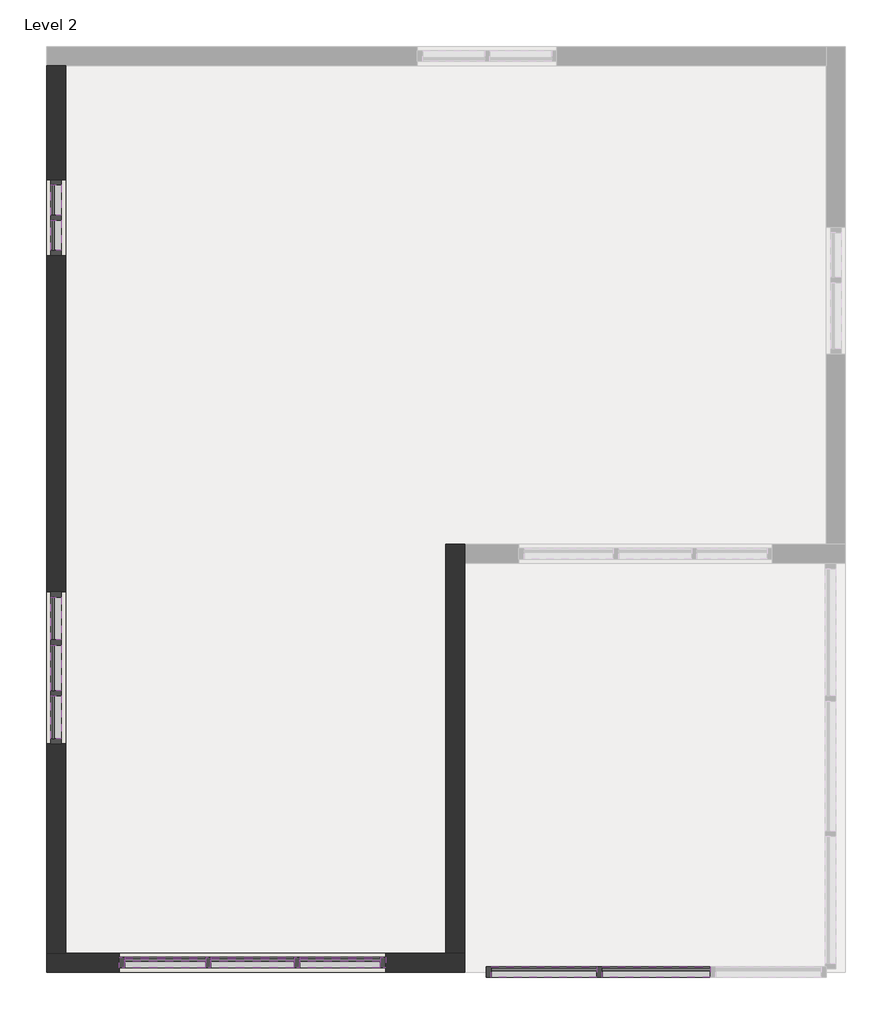
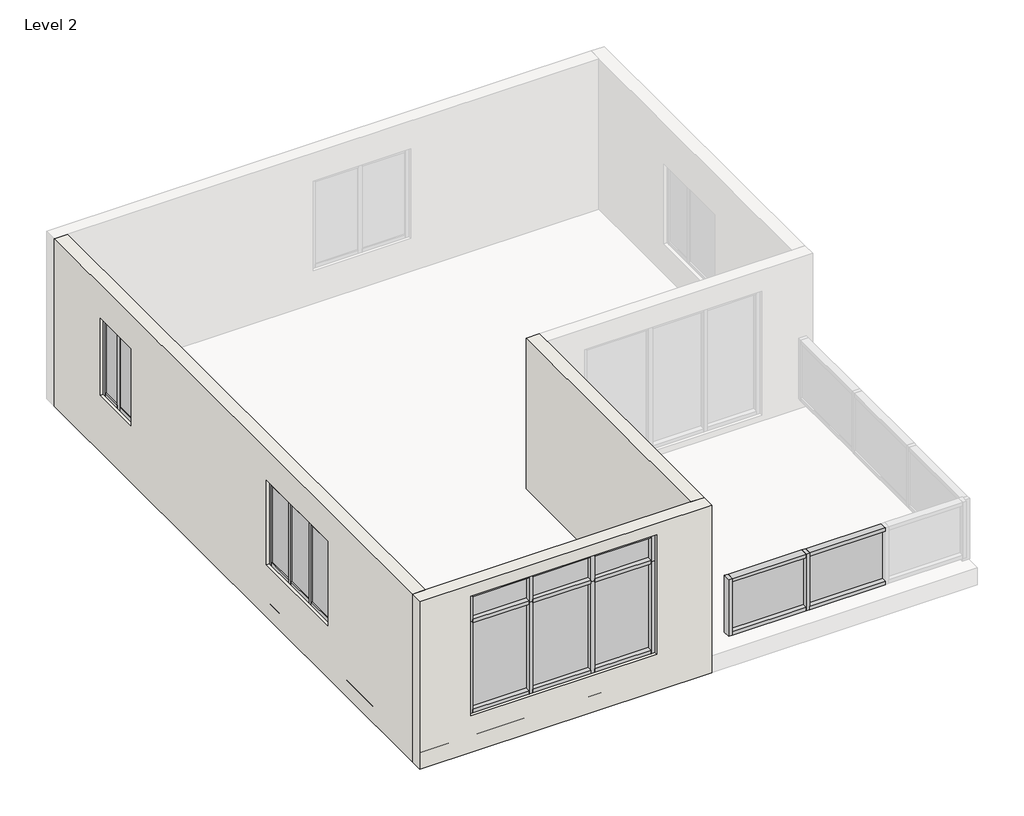
# One storey, part 1 of 2: 40 members, 13 plates, 3 walls.
"""IFC4 building model written with IfcOpenShell, lengths in millimetres."""

from ifc_helpers import new_model, si_unit, frame, origin, place, context, project, spatial, polyline, outline, extrude, faceted_brep, transform, mapped, element, save
from components import member_801a2072, member_cfcad22e, member_88aa5c81, member_7fa3b085, member_b06f4f27, member_562a4c76, member_90750a43, member_7fd687a9, member_02f15020, member_eb359e9e, member_20160837, member_9a0024e4, member_843225dc, member_b1264396, member_66888762, member_0b7646a3, member_a980948f, member_a8b9c919, member_bc6c8480, system_panel_glazed_55aea4e3, system_panel_glazed_a32de224, system_panel_glazed_06453807, system_panel_glazed_9d2fc6ec, system_panel_glazed_6a79ef8b, system_panel_glazed_d7c040a5, system_panel_glazed_fc3a3408, system_panel_glazed_b96b1f03, system_panel_glazed_c8fc80f3

model = new_model("IFC4")

# Units and contexts
model_context = context("Model", 3, world=origin())
ifc_project = project(units=[si_unit("LENGTHUNIT", "METRE", prefix="MILLI")], contexts=[model_context])

# Site, building, storey
site = spatial("IfcSite", under=ifc_project)
building = spatial("IfcBuilding", under=site)
storey = spatial("IfcBuildingStorey", under=building, Name="Level 2", Elevation=3048.0)

# Members
placement = place(None, origin())
member_shape = member_801a2072(model_context)
element("IfcMember", 1, ObjectType="Rectangular Mullion : 2.5\" x 5\" rectangular", at=placement, inside=storey, context=model_context, shape_type="MappedRepresentation", body=[
    mapped(member_shape, transform((-14543.6018575, -15040.4378384, 3718.9773685), x_axis=(0.0, 0.0, -1.0), y_axis=(0.0, -1.0, 0.0), z_axis=(-1.0, 0.0, 0.0))),
])
element("IfcMember", 2, ObjectType="Rectangular Mullion : 2.5\" x 5\" rectangular", at=placement, inside=storey, context=model_context, shape_type="MappedRepresentation", body=[
    mapped(member_shape, transform((-16645.4518575, -15040.4378384, 3718.9773685), x_axis=(0.0, 0.0, -1.0), y_axis=(0.0, -1.0, 0.0), z_axis=(-1.0, 0.0, 0.0))),
])
member_2_shape = member_cfcad22e(model_context)
element("IfcMember", 3, ObjectType="Rectangular Mullion : 2.5\" x 5\" rectangular", at=placement, inside=storey, context=model_context, shape_type="MappedRepresentation", body=[
    mapped(member_2_shape, transform((-15610.4018575, -15040.4378384, 3718.9773685), x_axis=(0.0, 0.0, -1.0), y_axis=(0.0, -1.0, 0.0), z_axis=(-1.0, 0.0, 0.0))),
])
element("IfcMember", 4, ObjectType="Rectangular Mullion : 2.5\" x 5\" rectangular", at=placement, inside=storey, context=model_context, shape_type="MappedRepresentation", body=[
    mapped(member_2_shape, transform((-14607.1018575, -15040.4378384, 5895.6635035), x_axis=(0.0, 0.0, 1.0), y_axis=(0.0, -1.0, 0.0), z_axis=(1.0, 0.0, 0.0))),
])
element("IfcMember", 5, ObjectType="Rectangular Mullion : 2.5\" x 5\" rectangular", at=placement, inside=storey, context=model_context, shape_type="MappedRepresentation", body=[
    mapped(member_shape, transform((-15673.9018575, -15040.4378384, 5895.6635035), x_axis=(0.0, 0.0, 1.0), y_axis=(0.0, -1.0, 0.0), z_axis=(1.0, 0.0, 0.0))),
])
element("IfcMember", 6, ObjectType="Rectangular Mullion : 2.5\" x 5\" rectangular", at=placement, inside=storey, context=model_context, shape_type="MappedRepresentation", body=[
    mapped(member_shape, transform((-13572.0518575, -15040.4378384, 5895.6635035), x_axis=(0.0, 0.0, 1.0), y_axis=(0.0, -1.0, 0.0), z_axis=(1.0, 0.0, 0.0))),
])
member_3_shape = member_88aa5c81(model_context)
element("IfcMember", 7, ObjectType="Rectangular Mullion : 2.5\" x 5\" rectangular", at=placement, inside=storey, context=model_context, shape_type="MappedRepresentation", body=[
    mapped(member_3_shape, transform((-13572.0518575, -15040.4378384, 5387.6635035), x_axis=(0.0, 0.0, 1.0), y_axis=(0.0, -1.0, 0.0), z_axis=(1.0, 0.0, 0.0))),
])
element("IfcMember", 8, ObjectType="Rectangular Mullion : 2.5\" x 5\" rectangular", at=placement, inside=storey, context=model_context, shape_type="MappedRepresentation", body=[
    mapped(member_3_shape, transform((-15673.9018575, -15040.4378384, 5387.6635035), x_axis=(0.0, 0.0, 1.0), y_axis=(0.0, -1.0, 0.0), z_axis=(1.0, 0.0, 0.0))),
])
member_4_shape = member_7fa3b085(model_context)
element("IfcMember", 9, ObjectType="Rectangular Mullion : 2.5\" x 5\" rectangular", at=placement, inside=storey, context=model_context, shape_type="MappedRepresentation", body=[
    mapped(member_4_shape, transform((-14607.1018575, -15040.4378384, 5387.6635035), x_axis=(0.0, 0.0, 1.0), y_axis=(0.0, -1.0, 0.0), z_axis=(1.0, 0.0, 0.0))),
])
member_5_shape = member_b06f4f27(model_context)
element("IfcMember", 10, ObjectType="Rectangular Mullion : 2.5\" x 5\" rectangular", at=placement, inside=storey, context=model_context, shape_type="MappedRepresentation", body=[
    mapped(member_5_shape, transform((-15642.1518575, -15040.4378384, 3718.9773685), x_axis=(1.0, 0.0, 0.0), y_axis=(0.0, -1.0, 0.0), z_axis=(0.0, 0.0, -1.0))),
])
element("IfcMember", 11, ObjectType="Rectangular Mullion : 2.5\" x 5\" rectangular", at=placement, inside=storey, context=model_context, shape_type="MappedRepresentation", body=[
    mapped(member_5_shape, transform((-14575.3518575, -15040.4378384, 3718.9773685), x_axis=(1.0, 0.0, 0.0), y_axis=(0.0, -1.0, 0.0), z_axis=(0.0, 0.0, -1.0))),
])
member_6_shape = member_562a4c76(model_context)
element("IfcMember", 12, ObjectType="Rectangular Mullion : 2.5\" x 5\" rectangular", at=placement, inside=storey, context=model_context, shape_type="MappedRepresentation", body=[
    mapped(member_6_shape, transform((-16708.9518575, -15040.4378384, 5387.6635035), x_axis=(-1.0, 0.0, 0.0), y_axis=(0.0, -1.0, 0.0), z_axis=(0.0, 0.0, 1.0))),
])
element("IfcMember", 13, ObjectType="Rectangular Mullion : 2.5\" x 5\" rectangular", at=placement, inside=storey, context=model_context, shape_type="MappedRepresentation", body=[
    mapped(member_6_shape, transform((-13508.5518575, -15040.4378384, 3718.9773685), x_axis=(1.0, 0.0, 0.0), y_axis=(0.0, -1.0, 0.0), z_axis=(0.0, 0.0, -1.0))),
])
member_7_shape = member_90750a43(model_context)
element("IfcMember", 14, ObjectType="Rectangular Mullion : 2.5\" x 5\" rectangular", at=placement, inside=storey, context=model_context, shape_type="MappedRepresentation", body=[
    mapped(member_7_shape, transform((-15642.1518575, -15040.4378384, 5387.6635035), x_axis=(1.0, 0.0, 0.0), y_axis=(0.0, -1.0, 0.0), z_axis=(0.0, 0.0, -1.0))),
])
element("IfcMember", 15, ObjectType="Rectangular Mullion : 2.5\" x 5\" rectangular", at=placement, inside=storey, context=model_context, shape_type="MappedRepresentation", body=[
    mapped(member_7_shape, transform((-14575.3518575, -15040.4378384, 5387.6635035), x_axis=(1.0, 0.0, 0.0), y_axis=(0.0, -1.0, 0.0), z_axis=(0.0, 0.0, -1.0))),
])
member_8_shape = member_7fd687a9(model_context)
element("IfcMember", 16, ObjectType="Rectangular Mullion : 2.5\" x 5\" rectangular", at=placement, inside=storey, context=model_context, shape_type="MappedRepresentation", body=[
    mapped(member_8_shape, transform((-16708.9518575, -15040.4378384, 5895.6635035), x_axis=(-1.0, 0.0, 0.0), y_axis=(0.0, -1.0, 0.0), z_axis=(0.0, 0.0, 1.0))),
])
element("IfcMember", 17, ObjectType="Rectangular Mullion : 2.5\" x 5\" rectangular", at=placement, inside=storey, context=model_context, shape_type="MappedRepresentation", body=[
    mapped(member_8_shape, transform((-13508.5518575, -15040.4378384, 5387.6635035), x_axis=(1.0, 0.0, 0.0), y_axis=(0.0, -1.0, 0.0), z_axis=(0.0, 0.0, -1.0))),
])
member_9_shape = member_02f15020(model_context)
element("IfcMember", 18, ObjectType="Rectangular Mullion : 2.5\" x 5\" rectangular", at=placement, inside=storey, context=model_context, shape_type="MappedRepresentation", body=[
    mapped(member_9_shape, transform((-12302.0518575, -15154.7378384, 4689.3272807), x_axis=(-1.0, 0.0, 0.0), y_axis=(0.0, -1.0, 0.0), z_axis=(0.0, 0.0, 1.0))),
])
member_10_shape = member_eb359e9e(model_context)
element("IfcMember", 19, ObjectType="Rectangular Mullion : 2.5\" x 5\" rectangular", at=placement, inside=storey, context=model_context, shape_type="MappedRepresentation", body=[
    mapped(member_10_shape, transform((-10970.6685242, -15154.7378384, 4689.3272807), x_axis=(0.0, 0.0, 1.0), y_axis=(0.0, -1.0, 0.0), z_axis=(1.0, 0.0, 0.0))),
])
element("IfcMember", 20, ObjectType="Rectangular Mullion : 2.5\" x 5\" rectangular", at=placement, inside=storey, context=model_context, shape_type="MappedRepresentation", body=[
    mapped(member_10_shape, transform((-12238.5518575, -15154.7378384, 3657.6), x_axis=(0.0, 0.0, -1.0), y_axis=(0.0, -1.0, 0.0), z_axis=(-1.0, 0.0, 0.0))),
])
member_11_shape = member_20160837(model_context)
element("IfcMember", 21, ObjectType="Rectangular Mullion : 2.5\" x 5\" rectangular", at=placement, inside=storey, context=model_context, shape_type="MappedRepresentation", body=[
    mapped(member_11_shape, transform((-10938.9185242, -15154.7378384, 3657.6), x_axis=(1.0, 0.0, 0.0), y_axis=(0.0, -1.0, 0.0), z_axis=(0.0, 0.0, -1.0))),
])
member_12_shape = member_9a0024e4(model_context)
element("IfcMember", 22, ObjectType="Rectangular Mullion : 2.5\" x 5\" rectangular", at=placement, inside=storey, context=model_context, shape_type="MappedRepresentation", body=[
    mapped(member_12_shape, transform((-9607.5351909, -15154.7378384, 4689.3272807), x_axis=(0.0, 0.0, 1.0), y_axis=(0.0, -1.0, 0.0), z_axis=(1.0, 0.0, 0.0))),
])
element("IfcMember", 23, ObjectType="Rectangular Mullion : 2.5\" x 5\" rectangular", at=placement, inside=storey, context=model_context, shape_type="MappedRepresentation", body=[
    mapped(member_12_shape, transform((-10907.1685242, -15154.7378384, 3657.6), x_axis=(0.0, 0.0, -1.0), y_axis=(0.0, -1.0, 0.0), z_axis=(-1.0, 0.0, 0.0))),
])
member_13_shape = member_843225dc(model_context)
element("IfcMember", 24, ObjectType="Rectangular Mullion : 2.5\" x 5\" rectangular", at=placement, inside=storey, context=model_context, shape_type="MappedRepresentation", body=[
    mapped(member_13_shape, transform((-17470.9518575, -6118.6878384, 5486.4886687), x_axis=(0.0, 0.0, 1.0), y_axis=(1.0, 0.0, 0.0), z_axis=(0.0, 1.0, 0.0))),
])
element("IfcMember", 25, ObjectType="Rectangular Mullion : 2.5\" x 5\" rectangular", at=placement, inside=storey, context=model_context, shape_type="MappedRepresentation", body=[
    mapped(member_13_shape, transform((-17470.9518575, -5693.2378384, 5486.4886687), x_axis=(0.0, 0.0, 1.0), y_axis=(1.0, 0.0, 0.0), z_axis=(0.0, 1.0, 0.0))),
])
member_14_shape = member_b1264396(model_context)
element("IfcMember", 26, ObjectType="Rectangular Mullion : 2.5\" x 5\" rectangular", at=placement, inside=storey, context=model_context, shape_type="MappedRepresentation", body=[
    mapped(member_14_shape, transform((-17470.9518575, -6086.9378384, 4077.6512698), x_axis=(0.0, 1.0, 0.0), y_axis=(1.0, 0.0, 0.0), z_axis=(0.0, 0.0, -1.0))),
])
element("IfcMember", 27, ObjectType="Rectangular Mullion : 2.5\" x 5\" rectangular", at=placement, inside=storey, context=model_context, shape_type="MappedRepresentation", body=[
    mapped(member_13_shape, transform((-17470.9518575, -6055.1878384, 4077.6512698), x_axis=(0.0, 0.0, -1.0), y_axis=(1.0, 0.0, 0.0), z_axis=(0.0, -1.0, 0.0))),
])
element("IfcMember", 28, ObjectType="Rectangular Mullion : 2.5\" x 5\" rectangular", at=placement, inside=storey, context=model_context, shape_type="MappedRepresentation", body=[
    mapped(member_13_shape, transform((-17470.9518575, -6480.6378384, 4077.6512698), x_axis=(0.0, 0.0, -1.0), y_axis=(1.0, 0.0, 0.0), z_axis=(0.0, -1.0, 0.0))),
])
member_15_shape = member_66888762(model_context)
element("IfcMember", 29, ObjectType="Rectangular Mullion : 2.5\" x 5\" rectangular", at=placement, inside=storey, context=model_context, shape_type="MappedRepresentation", body=[
    mapped(member_15_shape, transform((-17470.9518575, -6544.1378384, 5486.4886687), x_axis=(0.0, -1.0, 0.0), y_axis=(1.0, 0.0, 0.0), z_axis=(0.0, 0.0, 1.0))),
])
element("IfcMember", 30, ObjectType="Rectangular Mullion : 2.5\" x 5\" rectangular", at=placement, inside=storey, context=model_context, shape_type="MappedRepresentation", body=[
    mapped(member_15_shape, transform((-17470.9518575, -5629.7378384, 4077.6512698), x_axis=(0.0, 1.0, 0.0), y_axis=(1.0, 0.0, 0.0), z_axis=(0.0, 0.0, -1.0))),
])
member_16_shape = member_0b7646a3(model_context)
element("IfcMember", 31, ObjectType="Rectangular Mullion : 2.5\" x 5\" rectangular", at=placement, inside=storey, context=model_context, shape_type="MappedRepresentation", body=[
    mapped(member_16_shape, transform((-17470.9518575, -11833.6878384, 5535.6479327), x_axis=(0.0, 0.0, 1.0), y_axis=(1.0, 0.0, 0.0), z_axis=(0.0, 1.0, 0.0))),
])
element("IfcMember", 32, ObjectType="Rectangular Mullion : 2.5\" x 5\" rectangular", at=placement, inside=storey, context=model_context, shape_type="MappedRepresentation", body=[
    mapped(member_16_shape, transform((-17470.9518575, -10646.2378384, 5535.6479327), x_axis=(0.0, 0.0, 1.0), y_axis=(1.0, 0.0, 0.0), z_axis=(0.0, 1.0, 0.0))),
])
member_17_shape = member_a980948f(model_context)
element("IfcMember", 33, ObjectType="Rectangular Mullion : 2.5\" x 5\" rectangular", at=placement, inside=storey, context=model_context, shape_type="MappedRepresentation", body=[
    mapped(member_17_shape, transform((-17470.9518575, -11224.0878384, 5535.6479327), x_axis=(0.0, 0.0, 1.0), y_axis=(1.0, 0.0, 0.0), z_axis=(0.0, 1.0, 0.0))),
])
member_18_shape = member_a8b9c919(model_context)
element("IfcMember", 34, ObjectType="Rectangular Mullion : 2.5\" x 5\" rectangular", at=placement, inside=storey, context=model_context, shape_type="MappedRepresentation", body=[
    mapped(member_18_shape, transform((-17470.9518575, -11192.3378384, 3999.4214566), x_axis=(0.0, 1.0, 0.0), y_axis=(1.0, 0.0, 0.0), z_axis=(0.0, 0.0, -1.0))),
])
element("IfcMember", 35, ObjectType="Rectangular Mullion : 2.5\" x 5\" rectangular", at=placement, inside=storey, context=model_context, shape_type="MappedRepresentation", body=[
    mapped(member_18_shape, transform((-17470.9518575, -11801.9378384, 3999.4214566), x_axis=(0.0, 1.0, 0.0), y_axis=(1.0, 0.0, 0.0), z_axis=(0.0, 0.0, -1.0))),
])
element("IfcMember", 36, ObjectType="Rectangular Mullion : 2.5\" x 5\" rectangular", at=placement, inside=storey, context=model_context, shape_type="MappedRepresentation", body=[
    mapped(member_17_shape, transform((-17470.9518575, -11770.1878384, 3999.4214566), x_axis=(0.0, 0.0, -1.0), y_axis=(1.0, 0.0, 0.0), z_axis=(0.0, -1.0, 0.0))),
])
element("IfcMember", 37, ObjectType="Rectangular Mullion : 2.5\" x 5\" rectangular", at=placement, inside=storey, context=model_context, shape_type="MappedRepresentation", body=[
    mapped(member_16_shape, transform((-17470.9518575, -11160.5878384, 3999.4214566), x_axis=(0.0, 0.0, -1.0), y_axis=(1.0, 0.0, 0.0), z_axis=(0.0, -1.0, 0.0))),
])
element("IfcMember", 38, ObjectType="Rectangular Mullion : 2.5\" x 5\" rectangular", at=placement, inside=storey, context=model_context, shape_type="MappedRepresentation", body=[
    mapped(member_16_shape, transform((-17470.9518575, -12348.0378384, 3999.4214566), x_axis=(0.0, 0.0, -1.0), y_axis=(1.0, 0.0, 0.0), z_axis=(0.0, -1.0, 0.0))),
])
member_19_shape = member_bc6c8480(model_context)
element("IfcMember", 39, ObjectType="Rectangular Mullion : 2.5\" x 5\" rectangular", at=placement, inside=storey, context=model_context, shape_type="MappedRepresentation", body=[
    mapped(member_19_shape, transform((-17470.9518575, -12411.5378384, 5535.6479327), x_axis=(0.0, -1.0, 0.0), y_axis=(1.0, 0.0, 0.0), z_axis=(0.0, 0.0, 1.0))),
])
element("IfcMember", 40, ObjectType="Rectangular Mullion : 2.5\" x 5\" rectangular", at=placement, inside=storey, context=model_context, shape_type="MappedRepresentation", body=[
    mapped(member_19_shape, transform((-17470.9518575, -10582.7378384, 3999.4214566), x_axis=(0.0, 1.0, 0.0), y_axis=(1.0, 0.0, 0.0), z_axis=(0.0, 0.0, -1.0))),
])

# Plates
system_panel_glazed_shape = system_panel_glazed_55aea4e3(model_context)
element("IfcPlate", 41, ObjectType="System Panel : Glazed", at=placement, inside=storey, context=model_context, shape_type="MappedRepresentation", body=[
    mapped(system_panel_glazed_shape, transform((-16159.6768575, -15040.4378384, 3782.4773685), x_axis=(1.0, 0.0, 0.0), y_axis=(0.0, 1.0, 0.0), z_axis=(0.0, 0.0, 1.0))),
])
element("IfcPlate", 42, ObjectType="System Panel : Glazed", at=placement, inside=storey, context=model_context, shape_type="MappedRepresentation", body=[
    mapped(system_panel_glazed_shape, transform((-14057.8268575, -15040.4378384, 3782.4773685), x_axis=(1.0, 0.0, 0.0), y_axis=(0.0, 1.0, 0.0), z_axis=(0.0, 0.0, 1.0))),
])
system_panel_glazed_2_shape = system_panel_glazed_a32de224(model_context)
element("IfcPlate", 43, ObjectType="System Panel : Glazed", at=placement, inside=storey, context=model_context, shape_type="MappedRepresentation", body=[
    mapped(system_panel_glazed_2_shape, transform((-15108.7518575, -15040.4378384, 3782.4773685), x_axis=(1.0, 0.0, 0.0), y_axis=(0.0, 1.0, 0.0), z_axis=(0.0, 0.0, 1.0))),
])
system_panel_glazed_3_shape = system_panel_glazed_06453807(model_context)
element("IfcPlate", 44, ObjectType="System Panel : Glazed", at=placement, inside=storey, context=model_context, shape_type="MappedRepresentation", body=[
    mapped(system_panel_glazed_3_shape, transform((-16159.6768575, -15040.4378384, 5419.4135035), x_axis=(1.0, 0.0, 0.0), y_axis=(0.0, 1.0, 0.0), z_axis=(0.0, 0.0, 1.0))),
])
element("IfcPlate", 45, ObjectType="System Panel : Glazed", at=placement, inside=storey, context=model_context, shape_type="MappedRepresentation", body=[
    mapped(system_panel_glazed_3_shape, transform((-14057.8268575, -15040.4378384, 5419.4135035), x_axis=(1.0, 0.0, 0.0), y_axis=(0.0, 1.0, 0.0), z_axis=(0.0, 0.0, 1.0))),
])
system_panel_glazed_4_shape = system_panel_glazed_9d2fc6ec(model_context)
element("IfcPlate", 46, ObjectType="System Panel : Glazed", at=placement, inside=storey, context=model_context, shape_type="MappedRepresentation", body=[
    mapped(system_panel_glazed_4_shape, transform((-15108.7518575, -15040.4378384, 5419.4135035), x_axis=(1.0, 0.0, 0.0), y_axis=(0.0, 1.0, 0.0), z_axis=(0.0, 0.0, 1.0))),
])
system_panel_glazed_5_shape = system_panel_glazed_6a79ef8b(model_context)
element("IfcPlate", 47, ObjectType="System Panel : Glazed", at=placement, inside=storey, context=model_context, shape_type="MappedRepresentation", body=[
    mapped(system_panel_glazed_5_shape, transform((-11604.6101909, -15154.7378384, 3721.1), x_axis=(1.0, 0.0, 0.0), y_axis=(0.0, 1.0, 0.0), z_axis=(0.0, 0.0, 1.0))),
])
system_panel_glazed_6_shape = system_panel_glazed_d7c040a5(model_context)
element("IfcPlate", 48, ObjectType="System Panel : Glazed", at=placement, inside=storey, context=model_context, shape_type="MappedRepresentation", body=[
    mapped(system_panel_glazed_6_shape, transform((-10257.3518575, -15154.7378384, 3721.1), x_axis=(1.0, 0.0, 0.0), y_axis=(0.0, 1.0, 0.0), z_axis=(0.0, 0.0, 1.0))),
])
system_panel_glazed_7_shape = system_panel_glazed_fc3a3408(model_context)
element("IfcPlate", 49, ObjectType="System Panel : Glazed", at=placement, inside=storey, context=model_context, shape_type="MappedRepresentation", body=[
    mapped(system_panel_glazed_7_shape, transform((-17470.9518575, -6299.6628384, 4141.1512698), x_axis=(0.0, 1.0, 0.0), y_axis=(-1.0, 0.0, 0.0), z_axis=(0.0, 0.0, 1.0))),
])
element("IfcPlate", 50, ObjectType="System Panel : Glazed", at=placement, inside=storey, context=model_context, shape_type="MappedRepresentation", body=[
    mapped(system_panel_glazed_7_shape, transform((-17470.9518575, -5874.2128384, 4141.1512698), x_axis=(0.0, 1.0, 0.0), y_axis=(-1.0, 0.0, 0.0), z_axis=(0.0, 0.0, 1.0))),
])
system_panel_glazed_8_shape = system_panel_glazed_b96b1f03(model_context)
element("IfcPlate", 51, ObjectType="System Panel : Glazed", at=placement, inside=storey, context=model_context, shape_type="MappedRepresentation", body=[
    mapped(system_panel_glazed_8_shape, transform((-17470.9518575, -12090.8628384, 4062.9214566), x_axis=(0.0, 1.0, 0.0), y_axis=(-1.0, 0.0, 0.0), z_axis=(0.0, 0.0, 1.0))),
])
element("IfcPlate", 52, ObjectType="System Panel : Glazed", at=placement, inside=storey, context=model_context, shape_type="MappedRepresentation", body=[
    mapped(system_panel_glazed_8_shape, transform((-17470.9518575, -10903.4128384, 4062.9214566), x_axis=(0.0, 1.0, 0.0), y_axis=(-1.0, 0.0, 0.0), z_axis=(0.0, 0.0, 1.0))),
])
system_panel_glazed_9_shape = system_panel_glazed_c8fc80f3(model_context)
element("IfcPlate", 53, ObjectType="System Panel : Glazed", at=placement, inside=storey, context=model_context, shape_type="MappedRepresentation", body=[
    mapped(system_panel_glazed_9_shape, transform((-17470.9518575, -11497.1378384, 4062.9214566), x_axis=(0.0, 1.0, 0.0), y_axis=(-1.0, 0.0, 0.0), z_axis=(0.0, 0.0, 1.0))),
])

# Walls
element("IfcWall", 54, ObjectType="9\"", at=placement, inside=storey, context=model_context, shape_type="Brep", body=[
    faceted_brep([(-17585.2518575, -15154.7378384, 3048.0), (-12556.0518575, -15154.7378384, 3048.0), (-12556.0518575, -15154.7378384, 6096.0), (-17585.2518575, -15154.7378384, 6096.0), (-16708.9518575, -15154.7378384, 3718.9773685), (-16708.9518575, -15154.7378384, 5895.6635035), (-13508.5518575, -15154.7378384, 5895.6635035), (-13508.5518575, -15154.7378384, 3718.9773685), (-12556.0518575, -14926.1378384, 3048.0), (-12784.6518575, -14926.1378384, 3048.0), (-17356.6518575, -14926.1378384, 3048.0), (-17585.2518575, -14926.1378384, 3048.0), (-17585.2518575, -14926.1378384, 6096.0), (-17356.6518575, -14926.1378384, 6096.0), (-12784.6518575, -14926.1378384, 6096.0), (-12556.0518575, -14926.1378384, 6096.0), (-16708.9518575, -14926.1378384, 5895.6635035), (-16708.9518575, -14926.1378384, 3718.9773685), (-13508.5518575, -14926.1378384, 3718.9773685), (-13508.5518575, -14926.1378384, 5895.6635035)], [[[0, 1, 2, 3], [4, 5, 6, 7]], [[8, 9, 10, 11, 12, 13, 14, 15], [16, 17, 18, 19]], [[1, 0, 11, 10, 9, 8]], [[3, 2, 15, 14, 13, 12]], [[2, 1, 8, 15]], [[0, 3, 12, 11]], [[4, 17, 16, 5]], [[5, 16, 19, 6]], [[6, 19, 18, 7]], [[17, 4, 7, 18]]]),
])
element("IfcWall", 55, ObjectType="9\"", at=placement, inside=storey, context=model_context, shape_type="Brep", body=[
    faceted_brep([(-12556.0518575, -14926.1378384, 3048.0), (-12556.0518575, -10239.8378384, 3048.0), (-12556.0518575, -10011.2378384, 3048.0), (-12556.0518575, -10011.2378384, 6096.0), (-12556.0518575, -10239.8378384, 6096.0), (-12556.0518575, -14926.1378384, 6096.0), (-12784.6518575, -14926.1378384, 3048.0), (-12784.6518575, -14926.1378384, 6096.0), (-12784.6518575, -10011.2378384, 6096.0), (-12784.6518575, -10011.2378384, 3048.0)], [[[0, 1, 2, 3, 4, 5]], [[6, 7, 8, 9]], [[2, 1, 0, 6, 9]], [[5, 4, 3, 8, 7]], [[0, 5, 7, 6]], [[3, 2, 9, 8]]]),
])
element("IfcWall", 56, ObjectType="9\"", at=placement, inside=storey, context=model_context, shape_type="SweptSolid", body=[
    extrude(outline(polyline([(-4258.1378384, 3048.0), (-14926.1378384, 3048.0), (-14926.1378384, 6096.0), (-4258.1378384, 6096.0), (-4258.1378384, 3048.0)]), holes=[polyline([(-12411.5378384, 5535.6479327), (-12411.5378384, 3999.4214566), (-10582.7378384, 3999.4214566), (-10582.7378384, 5535.6479327), (-12411.5378384, 5535.6479327)]), polyline([(-6544.1378384, 5486.4886687), (-6544.1378384, 4077.6512698), (-5629.7378384, 4077.6512698), (-5629.7378384, 5486.4886687), (-6544.1378384, 5486.4886687)])]), frame((-17585.2518575, 0.0, 0.0), z_axis=(1.0, 0.0, 0.0), x_axis=(0.0, 1.0, 0.0)), (0.0, 0.0, 1.0), 228.6),
])

save(model, "model.ifc")

# Revit data of these elements
# Type "Rectangular Mullion : 2.5\" x 5\" rectangular"
#   built-in parameter 1007304 = 0.416667 (stored number, unit not read)
#   built-in parameter 1007301 = 0.104167 (stored number, unit not read)
#   built-in parameter 1007300 = 0.104167 (stored number, unit not read)
# Type "System Panel : Glazed"
#   Construction Type Id = "GSP4R"
#   Analytic Construction = "1/8 in Pilkington single glazing"
#   Visual Light Transmittance = 0.9
#   Solar Heat Gain Coefficient = 0.86
#   Heat Transfer Coefficient (U) = 1.18115 BTU/(h·ft²·°F)
#   Define Thermal Properties by = 1
# Type "9\""
#   Assembly Code = "B2010"
#   Layers, outside or top first: 0' - 9" no material (function 1)
# Elements 1, 2, 3, 4, 5, 6, 7, 8, 9, 10, 11, 12, 13, 14, 15, 16, 17, 18, 19, 20, 21, 22, 23, 24, 25, 26, 27, 28, 29, 30, 31, 32, 33, 34, 35, 36, 37, 38, 39, 40 (IfcMember, "Rectangular Mullion : 2.5\" x 5\" rectangular")
#   Phase Created = New Construction
#   Materials on its faces: "Aluminum"
# Elements 41, 42, 43, 44, 45, 46, 47, 48, 49, 50, 51, 52, 53 (IfcPlate, "System Panel : Glazed")
#   Phase Created = New Construction
#   Materials on its faces: "Glass"
# Elements 54, 55, 56 (IfcWall, "9\"")
#   Top Offset = 0' - 0"
#   Base Offset = 0' - 0"
#   Unconnected Height = 10' - 0"
#   wall height = 10' - 0"
#   Phase Created = New Construction
#   Base Constraint = Level 2
#   Materials on its faces: "Default Wall"
# Materials
#   "Aluminum": class "Metal", colour RGB 247 247 247, transparency 0, Description = "Aluminum 6061", Cost = 0
#   "Glass": class "Glass", colour RGB 0 128 192, transparency 0.75, Description = "Soda Lime Glass", Cost = 0
#   "Default Wall": colour RGB 128 128 128, transparency 0, Cost = 0
